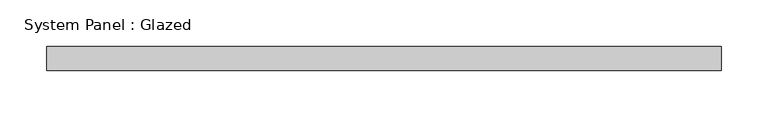
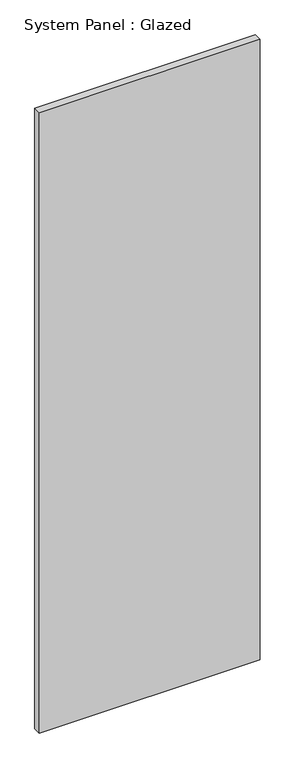
"""IFC4 building model written with IfcOpenShell, lengths in millimetres: plate geometry, System Panel : Glazed."""

from ifc_helpers import new_model, si_unit, origin, origin_with_axes, place, context, project, spatial, polyline, outline, extrude, source, transform, mapped, element, save


def system_panel_glazed_0ca22ccd(model_context):
    return source(origin(), model_context, "Body", "SweptSolid", [
        extrude(outline(polyline([(358.783438, 19.05), (-358.783438, 19.05), (-358.783438, 44.45), (358.783438, 44.45), (358.783438, 19.05)])), origin_with_axes(), (0.0, 0.0, 1.0), 2132.5340877),
    ])


if __name__ == "__main__":
    model = new_model("IFC4")
    model_context = context("Model", 3, world=origin())
    ifc_project = project(units=[si_unit("LENGTHUNIT", "METRE", prefix="MILLI")], contexts=[model_context])
    site = spatial("IfcSite", under=ifc_project)
    building = spatial("IfcBuilding", under=site)
    placement = place(None, origin())
    system_panel_glazed_shape = system_panel_glazed_0ca22ccd(model_context)
    element("IfcPlate", 1, ObjectType="System Panel : Glazed", at=placement, inside=building, context=model_context, shape_type="MappedRepresentation", body=[
        mapped(system_panel_glazed_shape, transform((0.0, 0.0, 0.0), x_axis=(1.0, 0.0, 0.0), y_axis=(0.0, 1.0, 0.0), z_axis=(0.0, 0.0, 1.0))),
    ])
    save(model, "model.ifc")

# Revit data of these elements
# Type "System Panel : Glazed"
#   Construction Type Id = "GSP4R"
#   Analytic Construction = "1/8 in Pilkington single glazing"
#   Visual Light Transmittance = 0.9
#   Solar Heat Gain Coefficient = 0.86
#   Heat Transfer Coefficient (U) = 1.18115 BTU/(h·ft²·°F)
# Element 1 (IfcPlate, "System Panel : Glazed")
#   Materials on its faces: "Glass"
# Materials
#   "Glass": class "Glass", colour RGB 0 128 192, transparency 0.75, Description = "Soda Lime Glass", Cost = 0
